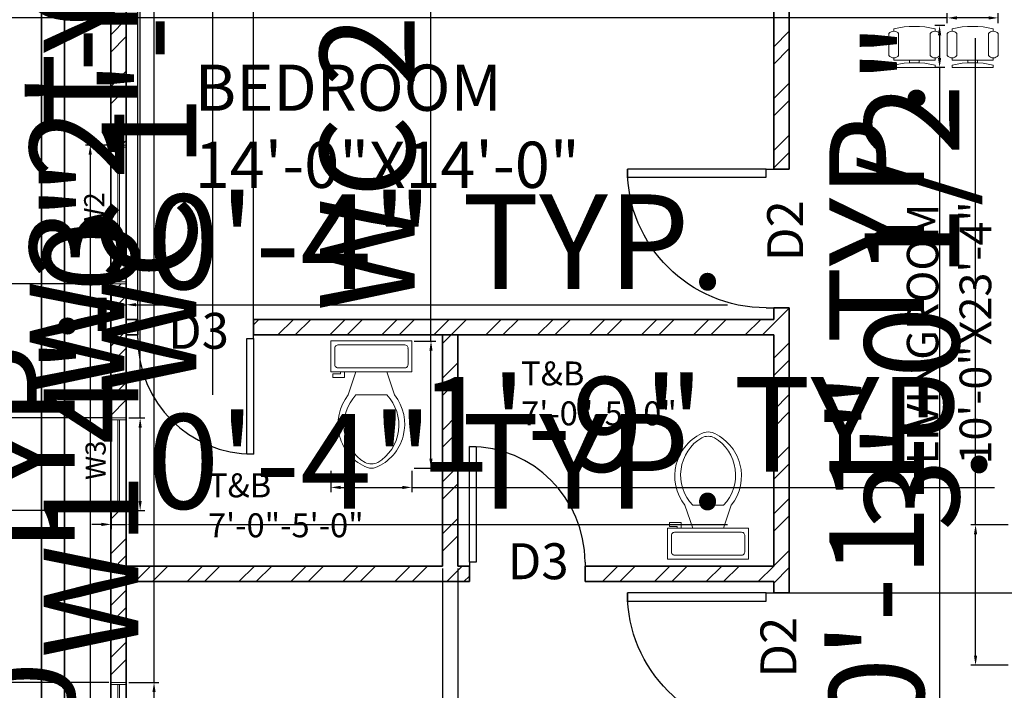
# Model space of a CAD drawing. Units: inches. Extents: x 1542 to 2523, y 1699 to 2449.
# Tile 3 of 7: x 1875 to 2130, y 1984 to 2158. Entities that reach past the tile are written whole.
import ezdxf

# ---------------------------------------------------------------- set-up
doc = ezdxf.new("R2010")
doc.units = ezdxf.units.IN
for name, color, linetype, lineweight in [('A-ANNO-DIMS', 7, 'Continuous', 18), ('A-ANNO-TEXT', 1, 'Continuous', 18), ('A-AREA-IDEN', 1, 'Continuous', 25), ('A-FLOR-FIXT', 9, 'Continuous', 18), ('A-WALL-PATT', 9, 'Continuous', 13), ('doors', 5, 'Continuous', 25), ('furniture', 9, 'Continuous', 18), ('walls', 7, 'Continuous', 35), ('windows', 93, 'Continuous', 18)]:
    doc.layers.add(name, color=color, linetype=linetype, lineweight=lineweight)
doc.styles.get("Standard").update_dxf_attribs({"font": 'arial.ttf'})
doc.dimstyles.new('ISO-25', dxfattribs={"dimtxt": 24.5625, "dimasz": 2.5, "dimexe": 1.25, "dimexo": 0.625, "dimtad": 1, "dimlunit": 4, "dimtxsty": 'Standard', "dimcen": 2.5, "dimadec": 0, "dimazin": 0, "dimtfac": 10, "dimtmove": 0, "dimatfit": 3, "dimfxl": 1, "dimarcsym": 0})

# ---------------------------------------------------------------- blocks, each defined once
blk = doc.blocks.new('*U2')
for p, q in [((0, 0), (0, -5)), ((30, 0), (30, -5))]:
    blk.add_line(p, q)
blk.add_lwpolyline([(0, 0), (0, 30), (1.75, 30), (1.75, 0)], close=True)
blk.add_arc((0, 0), 30, 0, 90)
blk = doc.blocks.new('Chair - Desk')
for p, q in [((-8.5, 0), (-8.5, -1)), ((-8.5, 0), (8.5, 0)), ((8.5, 0), (8.5, -1)), ((-8.5, -3), (-8.5, -4)), ((-8.5, -3), (8.5, -3)), ((-2, -3), (-2, -1.9355)), ((2, -1.9576), (2, -3)), ((8.5, -3), (8.5, -4)), ((-10.5, -5), (-10.5, -14)), ((-6.5, -14), (-6.5, -5)), ((6.5, -5), (6.5, -14)), ((10.5, -14), (10.5, -5)), ((-8.5, -15), (-8.5, -16)), ((8.5, -15), (8.5, -16))]:
    blk.add_line(p, q)
for centre, radius, start, end in [((-8.5, -6.5), 2.5, 36.8699, 143.1301), ((0, 34.625), 36.625, 256.5803, 283.4197), ((8.5, -6.5), 2.5, 36.8699, 143.1301), ((-8.5, -12.5), 2.5, 216.8699, 323.1301), ((0, 19.625), 36.625, 256.5803, 283.4197), ((8.5, -12.5), 2.5, 216.8699, 323.1301)]:
    blk.add_arc(centre, radius, start, end)
blk = doc.blocks.new('Toilet - top')
for p, q in [((9.5, -6), (9.5, -2)), ((-10, -8.5), (-8, -8.5)), ((-10, -9.5), (-10, -8.5)), ((-7, -9.5), (-10, -9.5)), ((-8, -8.5), (-8, -8)), ((-7, -8), (-7, -9.5)), ((-4, -8), (-6, -14)), ((4, -8), (6, -14)), ((4, -14), (-4, -14))]:
    blk.add_line(p, q)
blk.add_lwpolyline([(10.5, -8), (10.5, 0), (-10.5, 0), (-10.5, -8)], close=True)
for points in [[(-9.5, -2), (-9.5, -6)], [(8.5, -1), (-8.5, -1)], [(-8.5, -7), (8.5, -7)]]:
    blk.add_lwpolyline(points)
for centre, radius, start, end in [((-8.62, -1.88), 0.884, 81.8699, 188.1301), ((8.62, -1.88), 0.884, 351.8699, 98.1301), ((-8.62, -6.12), 0.884, 171.8699, 278.1301), ((8.62, -6.12), 0.884, 261.8699, 8.1301), ((3.52, -21.58), 12.17, 141.4691, 247.9714), ((4.2, -21.82), 11.33, 136.3677, 238.9468), ((-3.52, -21.58), 12.17, 292.0284, 38.5307), ((-4.2, -21.82), 11.33, 301.053, 43.6321), ((0, -27.88), 4, 245.7318, 294.2682), ((0, -29), 4, 254.8605, 285.1395)]:
    blk.add_arc(centre, radius, start, end)
blk = doc.blocks.new('WIN-W3-24IN')
for p, q in [((0, 0), (0, 24.03)), ((0, 24.03), (3.94, 24.03)), ((0, 23.53), (3.94, 23.53)), ((1.77, 0.5), (1.77, 23.53)), ((2.17, 0.5), (2.17, 23.53)), ((3.94, 24.03), (3.94, 0)), ((3.94, 0.5), (0, 0.5)), ((3.94, 0), (0, 0))]:
    blk.add_line(p, q)
blk = doc.blocks.new('WIN-W2-36IN')
for p, q in [((0, 3.94), (36.03, 3.94)), ((0, 0), (0, 3.94)), ((0.5, 0), (0.5, 3.94)), ((35.53, 3.94), (35.53, 0)), ((36.03, 3.94), (36.03, 0)), ((36.03, 0), (0, 0)), ((0.5, 2.17), (35.53, 2.17)), ((0.5, 1.77), (35.53, 1.77))]:
    blk.add_line(p, q)
blk = doc.blocks.new('WIN-W1-48IN')
for p, q in [((0, 0), (0, 48.03)), ((0, 48.03), (3.94, 48.03)), ((0, 47.53), (3.94, 47.53)), ((1.77, 0.5), (1.77, 47.53)), ((2.17, 0.5), (2.17, 47.53)), ((3.94, 48.03), (3.94, 0)), ((3.94, 0.5), (0, 0.5)), ((3.94, 0), (0, 0))]:
    blk.add_line(p, q)
blk = doc.blocks.new('*D26')
at = {"layer": 'A-ANNO-DIMS', "color": 0, "lineweight": -2, "transparency": 16777216}
for p, q in [((2115.34, 2158.69), (1845.86, 2158.69)), ((2115.34, 2157.33), (2115.34, 2159.94)), ((2126.05, 2158.69), (2117.84, 2158.69)), ((2128.55, 2157.33), (2128.55, 2159.94))]:
    blk.add_line(p, q, dxfattribs=at)
at = {"layer": 'A-ANNO-DIMS', "color": 0, "transparency": 16777216}
for points in [[(2117.84, 2159.1), (2117.84, 2158.27), (2115.34, 2158.69)], [(2126.05, 2159.1), (2126.05, 2158.27), (2128.55, 2158.69)]]:
    blk.add_solid(points, dxfattribs=at)
at = {"layer": 'Defpoints', "color": 0, "transparency": 16777216}
for p in [(2115.34, 2158.69), (2115.34, 2156.7), (2128.55, 2156.7)]:
    blk.add_point(p, dxfattribs=at)
at = {"layer": 'A-ANNO-DIMS', "color": 0, "transparency": 16777216, "insert": (1979.35, 2172.01), "char_height": 24.5625, "attachment_point": 5}
blk.add_mtext('CHAIR 1\'-1" TYP.', dxfattribs=at)
blk = doc.blocks.new('*D27')
at = {"layer": 'A-ANNO-DIMS', "color": 0, "lineweight": -2, "transparency": 16777216}
for p, q in [((2114.72, 2156.7), (2112.11, 2156.7)), ((2113.36, 2154.2), (2113.36, 2148.3)), ((2114.72, 2145.8), (2112.11, 2145.8)), ((2113.36, 2145.8), (2113.36, 1973.25))]:
    blk.add_line(p, q, dxfattribs=at)
at = {"layer": 'A-ANNO-DIMS', "color": 0, "transparency": 16777216}
for points in [[(2112.94, 2154.2), (2113.78, 2154.2), (2113.36, 2156.7)], [(2112.94, 2148.3), (2113.78, 2148.3), (2113.36, 2145.8)]]:
    blk.add_solid(points, dxfattribs=at)
at = {"layer": 'Defpoints', "color": 0, "transparency": 16777216}
for p in [(2115.34, 2156.7), (2113.36, 2145.8), (2115.34, 2145.8)]:
    blk.add_point(p, dxfattribs=at)
at = {"layer": 'A-ANNO-DIMS', "color": 0, "transparency": 16777216, "insert": (2100.19, 2058.28), "char_height": 24.5625, "attachment_point": 5, "rotation": 90}
blk.add_mtext('0\'-11" TYP.', dxfattribs=at)
blk = doc.blocks.new('*D28')
at = {"layer": 'A-ANNO-DIMS', "color": 0, "lineweight": -2, "transparency": 16777216}
for p, q in [((1905.99, 2054.87), (1905.99, 2270.35)), ((1903.01, 2054.87), (1907.24, 2054.87)), ((1905.99, 2033.33), (1905.99, 2052.37)), ((1903.01, 2030.83), (1907.24, 2030.83))]:
    blk.add_line(p, q, dxfattribs=at)
at = {"layer": 'A-ANNO-DIMS', "color": 0, "transparency": 16777216}
for points in [[(1905.57, 2052.37), (1906.4, 2052.37), (1905.99, 2054.87)], [(1905.57, 2033.33), (1906.4, 2033.33), (1905.99, 2030.83)]]:
    blk.add_solid(points, dxfattribs=at)
at = {"layer": 'Defpoints', "color": 0, "transparency": 16777216}
for p in [(1902.38, 2054.87), (1905.99, 2054.87), (1902.38, 2030.83)]:
    blk.add_point(p, dxfattribs=at)
at = {"layer": 'A-ANNO-DIMS', "color": 0, "transparency": 16777216, "insert": (1892.81, 2163.86), "char_height": 24.5625, "attachment_point": 5, "rotation": 90}
blk.add_mtext('W3 2\'-0" TYP.', dxfattribs=at)
blk = doc.blocks.new('*D29')
at = {"layer": 'A-ANNO-DIMS', "color": 0, "lineweight": -2, "transparency": 16777216}
for p, q in [((1898.45, 2030.21), (1898.45, 2025.98)), ((1902.38, 2030.21), (1902.38, 2025.98)), ((1895.95, 2027.23), (1893.45, 2027.23)), ((1898.45, 2027.23), (1902.38, 2027.23)), ((1904.88, 2027.23), (2058.35, 2027.23))]:
    blk.add_line(p, q, dxfattribs=at)
at = {"layer": 'A-ANNO-DIMS', "color": 0, "transparency": 16777216}
for points in [[(1895.95, 2027.65), (1895.95, 2026.81), (1898.45, 2027.23)], [(1904.88, 2027.65), (1904.88, 2026.81), (1902.38, 2027.23)]]:
    blk.add_solid(points, dxfattribs=at)
at = {"layer": 'Defpoints', "color": 0, "transparency": 16777216}
for p in [(1898.45, 2030.83), (1902.38, 2030.83), (1902.38, 2027.23)]:
    blk.add_point(p, dxfattribs=at)
at = {"layer": 'A-ANNO-DIMS', "color": 0, "transparency": 16777216, "insert": (1982.87, 2040.39), "char_height": 24.562, "attachment_point": 5}
blk.add_mtext('0\'-4" TYP.', dxfattribs=at)
blk = doc.blocks.new('*D30')
at = {"layer": 'A-ANNO-DIMS', "color": 0, "lineweight": -2, "transparency": 16777216}
for p, q in [((2181.19, 2203.89), (2176.38, 2203.89)), ((2177.63, 2201.39), (2177.63, 2178.49)), ((2181.19, 2175.99), (2176.38, 2175.99)), ((2177.63, 2175.99), (2177.63, 1878.93))]:
    blk.add_line(p, q, dxfattribs=at)
at = {"layer": 'A-ANNO-DIMS', "color": 0, "transparency": 16777216}
for points in [[(2177.21, 2201.39), (2178.05, 2201.39), (2177.63, 2203.89)], [(2177.21, 2178.49), (2178.05, 2178.49), (2177.63, 2175.99)]]:
    blk.add_solid(points, dxfattribs=at)
at = {"layer": 'Defpoints', "color": 0, "transparency": 16777216}
for p in [(2181.81, 2203.89), (2177.63, 2175.99), (2181.81, 2175.99)]:
    blk.add_point(p, dxfattribs=at)
at = {"layer": 'A-ANNO-DIMS', "color": 0, "transparency": 16777216, "insert": (2164.46, 2026.21), "char_height": 24.5625, "attachment_point": 5, "rotation": 90}
blk.add_mtext('TV UNIT 2\'-4" TYP.', dxfattribs=at)
blk = doc.blocks.new('*D32')
at = {"layer": 'A-ANNO-DIMS', "color": 0, "lineweight": -2, "transparency": 16777216}
for p, q in [((1922.46, 2274.54), (1926.04, 2274.54)), ((1924.79, 2272.04), (1924.79, 2257.33)), ((1922.46, 2254.83), (1926.04, 2254.83)), ((1924.79, 2254.83), (1924.79, 2060.84))]:
    blk.add_line(p, q, dxfattribs=at)
at = {"layer": 'A-ANNO-DIMS', "color": 0, "transparency": 16777216}
for points in [[(1924.37, 2272.04), (1925.21, 2272.04), (1924.79, 2274.54)], [(1924.37, 2257.33), (1925.21, 2257.33), (1924.79, 2254.83)]]:
    blk.add_solid(points, dxfattribs=at)
at = {"layer": 'Defpoints', "color": 0, "transparency": 16777216}
for p in [(1921.83, 2274.54), (1921.83, 2254.83), (1924.79, 2254.83)]:
    blk.add_point(p, dxfattribs=at)
at = {"layer": 'A-ANNO-DIMS', "color": 0, "transparency": 16777216, "insert": (1911.46, 2156.58), "char_height": 24.5625, "attachment_point": 5, "rotation": 90}
blk.add_mtext('WC 1\'-7 1/2"', dxfattribs=at)
blk = doc.blocks.new('*D34')
at = {"layer": 'A-ANNO-DIMS', "color": 0, "lineweight": -2, "transparency": 16777216}
for p, q in [((1981.43, 2074.83), (1981.43, 2296.01)), ((1977.09, 2074.83), (1982.68, 2074.83)), ((1981.43, 2044.29), (1981.43, 2072.33)), ((1977.09, 2041.79), (1982.68, 2041.79))]:
    blk.add_line(p, q, dxfattribs=at)
at = {"layer": 'A-ANNO-DIMS', "color": 0, "transparency": 16777216}
for points in [[(1981.01, 2072.33), (1981.84, 2072.33), (1981.43, 2074.83)], [(1981.01, 2044.29), (1981.84, 2044.29), (1981.43, 2041.79)]]:
    blk.add_solid(points, dxfattribs=at)
at = {"layer": 'Defpoints', "color": 0, "transparency": 16777216}
for p in [(1976.47, 2074.83), (1981.43, 2074.83), (1976.47, 2041.79)]:
    blk.add_point(p, dxfattribs=at)
at = {"layer": 'A-ANNO-DIMS', "color": 0, "transparency": 16777216, "insert": (1968.1, 2186.67), "char_height": 24.5625, "attachment_point": 5, "rotation": 90}
blk.add_mtext('WC 2\'-9" TYP.', dxfattribs=at)
blk = doc.blocks.new('*D35')
at = {"layer": 'A-ANNO-DIMS', "color": 0, "lineweight": -2, "transparency": 16777216}
for p, q in [((1955.47, 2041.16), (1955.47, 2035.58)), ((1976.47, 2041.16), (1976.47, 2035.58)), ((1957.97, 2036.83), (1973.97, 2036.83)), ((1976.47, 2036.83), (2127.63, 2036.83))]:
    blk.add_line(p, q, dxfattribs=at)
at = {"layer": 'A-ANNO-DIMS', "color": 0, "transparency": 16777216}
for points in [[(1957.97, 2037.25), (1957.97, 2036.41), (1955.47, 2036.83)], [(1973.97, 2037.25), (1973.97, 2036.41), (1976.47, 2036.83)]]:
    blk.add_solid(points, dxfattribs=at)
at = {"layer": 'Defpoints', "color": 0, "transparency": 16777216}
for p in [(1955.47, 2041.79), (1976.47, 2041.79), (1976.47, 2036.83)]:
    blk.add_point(p, dxfattribs=at)
at = {"layer": 'A-ANNO-DIMS', "color": 0, "transparency": 16777216, "insert": (2053.3, 2050), "char_height": 24.562, "attachment_point": 5}
blk.add_mtext('1\'-9" TYP.', dxfattribs=at)
blk = doc.blocks.new('*D36')
at = {"layer": 'A-ANNO-DIMS', "color": 0, "lineweight": -2, "transparency": 16777216}
for p, q in [((1897.82, 2125.68), (1891.79, 2125.68)), ((1893.04, 2123.18), (1893.04, 2092.15)), ((1897.82, 2089.65), (1891.79, 2089.65)), ((1893.04, 2089.65), (1893.04, 1874.17))]:
    blk.add_line(p, q, dxfattribs=at)
at = {"layer": 'A-ANNO-DIMS', "color": 0, "transparency": 16777216}
for points in [[(1892.62, 2123.18), (1893.46, 2123.18), (1893.04, 2125.68)], [(1892.62, 2092.15), (1893.46, 2092.15), (1893.04, 2089.65)]]:
    blk.add_solid(points, dxfattribs=at)
at = {"layer": 'Defpoints', "color": 0, "transparency": 16777216}
for p in [(1898.45, 2125.68), (1893.04, 2089.65), (1898.45, 2089.65)]:
    blk.add_point(p, dxfattribs=at)
at = {"layer": 'A-ANNO-DIMS', "color": 0, "transparency": 16777216, "insert": (1879.87, 1980.66), "char_height": 24.5625, "attachment_point": 5, "rotation": 90}
blk.add_mtext('W2 3\'-0" TYP.', dxfattribs=at)
blk = doc.blocks.new('*D37')
at = {"layer": 'A-ANNO-DIMS', "color": 0, "lineweight": -2, "transparency": 16777216}
for p, q in [((1898.45, 2089.02), (1898.45, 2082.99)), ((1902.38, 2089.02), (1902.38, 2082.99)), ((1895.95, 2084.24), (1893.45, 2084.24)), ((1898.45, 2084.24), (1902.38, 2084.24)), ((1904.88, 2084.24), (2058.35, 2084.24))]:
    blk.add_line(p, q, dxfattribs=at)
at = {"layer": 'A-ANNO-DIMS', "color": 0, "transparency": 16777216}
for points in [[(1895.95, 2084.66), (1895.95, 2083.83), (1898.45, 2084.24)], [(1904.88, 2084.66), (1904.88, 2083.83), (1902.38, 2084.24)]]:
    blk.add_solid(points, dxfattribs=at)
at = {"layer": 'Defpoints', "color": 0, "transparency": 16777216}
for p in [(1898.45, 2089.65), (1902.38, 2089.65), (1902.38, 2084.24)]:
    blk.add_point(p, dxfattribs=at)
at = {"layer": 'A-ANNO-DIMS', "color": 0, "transparency": 16777216, "insert": (1982.87, 2097.41), "char_height": 24.562, "attachment_point": 5}
blk.add_mtext('0\'-4" TYP.', dxfattribs=at)
blk = doc.blocks.new('*D40')
at = {"layer": 'A-ANNO-DIMS', "color": 0, "lineweight": -2, "transparency": 16777216}
for p, q in [((1909.59, 1986.22), (1909.59, 2201.7)), ((1903.01, 1986.22), (1910.84, 1986.22)), ((1909.59, 1940.69), (1909.59, 1983.72)), ((1903.01, 1938.19), (1910.84, 1938.19))]:
    blk.add_line(p, q, dxfattribs=at)
at = {"layer": 'A-ANNO-DIMS', "color": 0, "transparency": 16777216}
for points in [[(1909.17, 1983.72), (1910, 1983.72), (1909.59, 1986.22)], [(1909.17, 1940.69), (1910, 1940.69), (1909.59, 1938.19)]]:
    blk.add_solid(points, dxfattribs=at)
at = {"layer": 'Defpoints', "color": 0, "transparency": 16777216}
for p in [(1902.38, 1986.22), (1909.59, 1986.22), (1902.38, 1938.19)]:
    blk.add_point(p, dxfattribs=at)
at = {"layer": 'A-ANNO-DIMS', "color": 0, "transparency": 16777216, "insert": (1896.42, 2095.21), "char_height": 24.5625, "attachment_point": 5, "rotation": 90}
blk.add_mtext('W1 4\'-0" TYP.', dxfattribs=at)
blk = doc.blocks.new('*D43')
at = {"layer": 'A-ANNO-DIMS', "color": 0, "lineweight": -2, "transparency": 16777216}
for p, q in [((2122.69, 2027.16), (2122.69, 2153.42)), ((2131.12, 2027.16), (2121.44, 2027.16)), ((2122.69, 1993.17), (2122.69, 2024.66)), ((2131.12, 1990.67), (2121.44, 1990.67))]:
    blk.add_line(p, q, dxfattribs=at)
at = {"layer": 'A-ANNO-DIMS', "color": 0, "transparency": 16777216}
for points in [[(2122.28, 2024.66), (2123.11, 2024.66), (2122.69, 2027.16)], [(2122.28, 1993.17), (2123.11, 1993.17), (2122.69, 1990.67)]]:
    blk.add_solid(points, dxfattribs=at)
at = {"layer": 'Defpoints', "color": 0, "transparency": 16777216}
for p in [(2122.69, 2027.16), (2131.75, 2027.16), (2131.75, 1990.67)]:
    blk.add_point(p, dxfattribs=at)
at = {"layer": 'A-ANNO-DIMS', "color": 0, "transparency": 16777216, "insert": (2109.36, 2091.54), "char_height": 24.562, "attachment_point": 5, "rotation": 90}
blk.add_mtext('3\'-0 1/2"', dxfattribs=at)
blk = doc.blocks.new('*D47')
at = {"layer": 'A-ANNO-DIMS', "color": 0, "lineweight": -2, "transparency": 16777216}
for p, q in [((2268.83, 2009.44), (2268.83, 2078.47)), ((2071.01, 2009.44), (2270.08, 2009.44)), ((2268.83, 1975.94), (2268.83, 2006.94)), ((2071.01, 1973.44), (2270.08, 1973.44))]:
    blk.add_line(p, q, dxfattribs=at)
at = {"layer": 'A-ANNO-DIMS', "color": 0, "transparency": 16777216}
for points in [[(2268.42, 2006.94), (2269.25, 2006.94), (2268.83, 2009.44)], [(2268.42, 1975.94), (2269.25, 1975.94), (2268.83, 1973.44)]]:
    blk.add_solid(points, dxfattribs=at)
at = {"layer": 'Defpoints', "color": 0, "transparency": 16777216}
for p in [(2070.38, 2009.44), (2268.83, 2009.44), (2070.38, 1973.44)]:
    blk.add_point(p, dxfattribs=at)
at = {"layer": 'A-ANNO-DIMS', "color": 0, "transparency": 16777216, "insert": (2255.66, 2045.2), "char_height": 24.562, "attachment_point": 5, "rotation": 90}
blk.add_mtext('3\'-0"', dxfattribs=at)
blk = doc.blocks.new('*D48')
at = {"layer": 'A-ANNO-DIMS', "color": 0, "lineweight": -2, "transparency": 16777216}
for p, q in [((1905.38, 2077.06), (1905.38, 2320.14)), ((1935.38, 2077.06), (1935.38, 2320.14)), ((1907.88, 2318.89), (1932.88, 2318.89)), ((1935.38, 2318.89), (2004.84, 2318.89))]:
    blk.add_line(p, q, dxfattribs=at)
at = {"layer": 'A-ANNO-DIMS', "color": 0, "transparency": 16777216}
for points in [[(1907.88, 2319.31), (1907.88, 2318.47), (1905.38, 2318.89)], [(1932.88, 2319.31), (1932.88, 2318.47), (1935.38, 2318.89)]]:
    blk.add_solid(points, dxfattribs=at)
at = {"layer": 'Defpoints', "color": 0, "transparency": 16777216}
for p in [(1935.38, 2318.89), (1905.38, 2076.44), (1935.38, 2076.44)]:
    blk.add_point(p, dxfattribs=at)
at = {"layer": 'A-ANNO-DIMS', "color": 0, "transparency": 16777216, "insert": (1971.36, 2332.05), "char_height": 24.562, "attachment_point": 5}
blk.add_mtext('2\'-6"', dxfattribs=at)
blk = doc.blocks.new('*D49')
at = {"layer": 'A-ANNO-DIMS', "color": 0, "lineweight": -2, "transparency": 16777216}
for p, q in [((1851.93, 1958.44), (1851.93, 2027.9)), ((2157.76, 1958.44), (1850.68, 1958.44)), ((1851.93, 1936.94), (1851.93, 1955.94)), ((2157.76, 1934.44), (1850.68, 1934.44))]:
    blk.add_line(p, q, dxfattribs=at)
at = {"layer": 'A-ANNO-DIMS', "color": 0, "transparency": 16777216}
for points in [[(1851.52, 1955.94), (1852.35, 1955.94), (1851.93, 1958.44)], [(1851.52, 1936.94), (1852.35, 1936.94), (1851.93, 1934.44)]]:
    blk.add_solid(points, dxfattribs=at)
at = {"layer": 'Defpoints', "color": 0, "transparency": 16777216}
for p in [(1851.93, 1958.44), (2158.38, 1958.44), (2158.38, 1934.44)]:
    blk.add_point(p, dxfattribs=at)
at = {"layer": 'A-ANNO-DIMS', "color": 0, "transparency": 16777216, "insert": (1838.77, 1994.42), "char_height": 24.562, "attachment_point": 5, "rotation": 90}
blk.add_mtext('2\'-0"', dxfattribs=at)
blk = doc.blocks.new('*D56')
at = {"layer": 'A-ANNO-DIMS', "color": 0, "lineweight": -2, "transparency": 16777216}
for p, q in [((1851.93, 2030.83), (1851.93, 2157.09)), ((1897.82, 2030.83), (1850.68, 2030.83)), ((1851.93, 1988.72), (1851.93, 2028.33)), ((1897.82, 1986.22), (1850.68, 1986.22))]:
    blk.add_line(p, q, dxfattribs=at)
at = {"layer": 'A-ANNO-DIMS', "color": 0, "transparency": 16777216}
for points in [[(1851.52, 2028.33), (1852.35, 2028.33), (1851.93, 2030.83)], [(1851.52, 1988.72), (1852.35, 1988.72), (1851.93, 1986.22)]]:
    blk.add_solid(points, dxfattribs=at)
at = {"layer": 'Defpoints', "color": 0, "transparency": 16777216}
for p in [(1851.93, 2030.83), (1898.45, 2030.83), (1898.45, 1986.22)]:
    blk.add_point(p, dxfattribs=at)
at = {"layer": 'A-ANNO-DIMS', "color": 0, "transparency": 16777216, "insert": (1838.6, 2095.21), "char_height": 24.562, "attachment_point": 5, "rotation": 90}
blk.add_mtext('3\'-8 1/2"', dxfattribs=at)
blk = doc.blocks.new('*D57')
at = {"layer": 'A-ANNO-DIMS', "color": 0, "lineweight": -2, "transparency": 16777216}
for p, q in [((1851.93, 2089.65), (1851.93, 2178.19)), ((1897.82, 2089.65), (1850.68, 2089.65)), ((1851.93, 2057.37), (1851.93, 2087.15)), ((1897.82, 2054.87), (1850.68, 2054.87))]:
    blk.add_line(p, q, dxfattribs=at)
at = {"layer": 'A-ANNO-DIMS', "color": 0, "transparency": 16777216}
for points in [[(1851.52, 2087.15), (1852.35, 2087.15), (1851.93, 2089.65)], [(1851.52, 2057.37), (1852.35, 2057.37), (1851.93, 2054.87)]]:
    blk.add_solid(points, dxfattribs=at)
at = {"layer": 'Defpoints', "color": 0, "transparency": 16777216}
for p in [(1851.93, 2089.65), (1898.45, 2089.65), (1898.45, 2054.87)]:
    blk.add_point(p, dxfattribs=at)
at = {"layer": 'A-ANNO-DIMS', "color": 0, "transparency": 16777216, "insert": (1838.98, 2135.17), "char_height": 24.562, "attachment_point": 5, "rotation": 90}
blk.add_mtext('2\'-11"', dxfattribs=at)
blk = doc.blocks.new('*D67')
at = {"layer": 'A-ANNO-DIMS', "color": 0, "lineweight": -2, "transparency": 16777216}
for p, q in [((1984.38, 2015.81), (1984.38, 1720.74)), ((1902.38, 2011.81), (1902.38, 1720.74)), ((1904.88, 1721.99), (1981.88, 1721.99)), ((1984.38, 1721.99), (2072.64, 1721.99))]:
    blk.add_line(p, q, dxfattribs=at)
at = {"layer": 'A-ANNO-DIMS', "color": 0, "transparency": 16777216}
for points in [[(1904.88, 1722.41), (1904.88, 1721.57), (1902.38, 1721.99)], [(1981.88, 1722.41), (1981.88, 1721.57), (1984.38, 1721.99)]]:
    blk.add_solid(points, dxfattribs=at)
at = {"layer": 'Defpoints', "color": 0, "transparency": 16777216}
for p in [(1984.38, 2016.44), (1902.38, 2012.44), (1984.38, 1721.99)]:
    blk.add_point(p, dxfattribs=at)
at = {"layer": 'A-ANNO-DIMS', "color": 0, "transparency": 16777216, "insert": (2029.76, 1735.15), "char_height": 24.562, "attachment_point": 5}
blk.add_mtext('6\'-10"', dxfattribs=at)
blk = doc.blocks.new('*D68')
at = {"layer": 'A-ANNO-DIMS', "color": 0, "lineweight": -2, "transparency": 16777216}
for p, q in [((1984.38, 2015.81), (1984.38, 1720.74)), ((1988.38, 2015.81), (1988.38, 1720.74)), ((1981.88, 1721.99), (1979.38, 1721.99)), ((1984.38, 1721.99), (1988.38, 1721.99)), ((1990.88, 1721.99), (2059.93, 1721.99))]:
    blk.add_line(p, q, dxfattribs=at)
at = {"layer": 'A-ANNO-DIMS', "color": 0, "transparency": 16777216}
for points in [[(1981.88, 1722.41), (1981.88, 1721.57), (1984.38, 1721.99)], [(1990.88, 1722.41), (1990.88, 1721.57), (1988.38, 1721.99)]]:
    blk.add_solid(points, dxfattribs=at)
at = {"layer": 'Defpoints', "color": 0, "transparency": 16777216}
for p in [(1984.38, 2016.44), (1988.38, 2016.44), (1988.38, 1721.99)]:
    blk.add_point(p, dxfattribs=at)
at = {"layer": 'A-ANNO-DIMS', "color": 0, "transparency": 16777216, "insert": (2026.65, 1735.15), "char_height": 24.562, "attachment_point": 5}
blk.add_mtext('0\'-4"', dxfattribs=at)
blk = doc.blocks.new('*D69')
at = {"layer": 'A-ANNO-DIMS', "color": 0, "lineweight": -2, "transparency": 16777216}
for p, q in [((1902.38, 2077.06), (1902.38, 2320.14)), ((1905.38, 2077.06), (1905.38, 2320.14)), ((1899.88, 2318.89), (1897.38, 2318.89)), ((1902.38, 2318.89), (1905.38, 2318.89)), ((1907.88, 2318.89), (1976.93, 2318.89))]:
    blk.add_line(p, q, dxfattribs=at)
at = {"layer": 'A-ANNO-DIMS', "color": 0, "transparency": 16777216}
for points in [[(1899.88, 2319.31), (1899.88, 2318.47), (1902.38, 2318.89)], [(1907.88, 2319.31), (1907.88, 2318.47), (1905.38, 2318.89)]]:
    blk.add_solid(points, dxfattribs=at)
at = {"layer": 'Defpoints', "color": 0, "transparency": 16777216}
for p in [(1905.38, 2318.89), (1902.38, 2076.44), (1905.38, 2076.44)]:
    blk.add_point(p, dxfattribs=at)
at = {"layer": 'A-ANNO-DIMS', "color": 0, "transparency": 16777216, "insert": (1943.65, 2332.06), "char_height": 24.562, "attachment_point": 5}
blk.add_mtext('0\'-3"', dxfattribs=at)

msp = doc.modelspace()

# ---------------------------------------------------------------- hatches: boundary and pattern name
at = {"layer": 'A-WALL-PATT'}
h = msp.add_hatch(dxfattribs=at)
h.set_pattern_fill('ANSI32', color=256)
h.paths.add_polyline_path([(1902.383, 2125.681), (1898.383, 2125.681), (1898.383, 2252.439), (2030.138, 2252.439), (2030.138, 2248.439), (1902.383, 2248.439)])
h = msp.add_hatch(dxfattribs=at)
h.set_pattern_fill('ANSI32', color=256)
h.paths.add_polyline_path([(2074.383, 2248.439), (2070.383, 2248.439), (2070.383, 2119.439), (2074.383, 2119.439)])
h = msp.add_hatch(dxfattribs=at)
h.set_pattern_fill('ANSI32', color=256)
h.paths.add_polyline_path([(1902.383, 2089.649), (1898.383, 2089.649), (1898.383, 2054.866), (1902.383, 2054.866)])
h = msp.add_hatch(dxfattribs=at)
h.set_pattern_fill('ANSI32', color=256)
h.paths.add_polyline_path([(2074.383, 2083.439), (2070.383, 2083.439), (2070.383, 2080.439), (1935.383, 2080.439), (1935.383, 2076.439), (2070.383, 2076.439), (2070.383, 2016.439), (2021.383, 2016.439), (2021.383, 2012.439), (2070.383, 2012.439), (2070.383, 2009.439), (2074.383, 2009.439), (2074.383, 2012.439)])
h = msp.add_hatch(dxfattribs=at)
h.set_pattern_fill('ANSI32', color=256)
h.paths.add_polyline_path([(1905.383, 2080.439), (1902.383, 2080.439), (1902.383, 2076.439), (1905.383, 2076.439)])
h = msp.add_hatch(dxfattribs=at)
h.set_pattern_fill('ANSI32', color=256)
h.paths.add_polyline_path([(1988.383, 2076.439), (1984.383, 2076.439), (1984.383, 2016.439), (1902.383, 2016.439), (1902.383, 2012.439), (1991.383, 2012.439), (1991.383, 2016.439), (1988.383, 2016.439)])
h = msp.add_hatch(dxfattribs=at)
h.set_pattern_fill('ANSI32', color=256)
h.paths.add_polyline_path([(1902.383, 2030.833), (1898.383, 2030.833), (1898.383, 1986.223), (1902.383, 1986.223)])

# ---------------------------------------------------------------- linework, layer by layer
at = {"layer": 'walls'}
for p, q in [((1880.383, 1750.439), (1880.383, 2290.439)), ((1886.383, 1756.439), (1886.383, 2284.439)), ((1898.383, 1840.439), (1898.383, 2252.439)), ((1902.383, 1844.439), (1902.383, 2248.439)), ((2070.383, 2119.439), (2070.383, 2248.439)), ((2074.383, 2119.439), (2074.383, 2248.439)), ((2070.383, 2119.439), (2074.383, 2119.439)), ((2074.383, 2083.439), (2070.383, 2083.439)), ((2070.383, 2080.439), (2070.383, 2083.439)), ((2074.383, 2080.439), (2074.383, 2083.439)), ((2074.383, 2009.439), (2074.383, 2083.439)), ((1902.383, 2080.439), (1905.383, 2080.439)), ((1905.383, 2080.439), (1902.383, 2080.439)), ((1905.383, 2080.439), (1905.383, 2076.439)), ((2070.383, 2080.439), (1935.383, 2080.439)), ((1935.383, 2076.439), (1935.383, 2080.439)), ((1905.383, 2076.439), (1902.383, 2076.439)), ((2070.383, 2076.439), (1935.383, 2076.439)), ((1984.383, 2016.439), (1984.383, 2076.439)), ((1988.383, 2016.439), (1988.383, 2076.439)), ((2070.383, 2016.439), (2070.383, 2076.439)), ((1984.383, 2016.439), (1902.383, 2016.439)), ((1988.383, 2016.439), (1991.383, 2016.439)), ((1991.383, 2016.439), (1988.383, 2016.439)), ((1991.383, 2016.439), (1991.383, 2012.439)), ((2070.383, 2016.439), (2021.383, 2016.439)), ((2021.383, 2012.439), (2021.383, 2016.439)), ((1991.383, 2012.439), (1902.383, 2012.439)), ((2070.383, 2012.439), (2021.383, 2012.439)), ((2070.383, 2009.439), (2070.383, 2012.439)), ((2074.383, 2012.439), (2074.383, 2009.439)), ((2074.383, 2009.439), (2070.383, 2009.439))]:
    msp.add_line(p, q, dxfattribs=at)

# ---------------------------------------------------------------- block references
at = {"layer": 'A-FLOR-FIXT'}
msp.add_blockref('Toilet - top', (1965.969, 2074.834), dxfattribs=at)
at = {"layer": 'A-FLOR-FIXT', "xscale": -1, "rotation": 180}
msp.add_blockref('Toilet - top', (2053.318, 2018.218), dxfattribs=at)
at = {"layer": 'doors', "xscale": -1.199999999999999, "yscale": 1.199999999999999, "zscale": 1.199999999999999, "rotation": 90}
for p in [(2068.383, 2119.439), (2068.383, 2009.439)]:
    msp.add_blockref('*U2', p, dxfattribs=at)
at = {"layer": 'doors', "rotation": 180}
msp.add_blockref('*U2', (1935.383, 2075.439), dxfattribs=at)
at = {"layer": 'doors'}
msp.add_blockref('*U2', (1991.383, 2017.439), dxfattribs=at)
at = {"layer": 'furniture', "xscale": 0.6288640780466365, "yscale": 0.6288640780466365, "zscale": 0.6288640780466365, "rotation": 180}
for p in [(2106.83, 2145.804), (2121.944, 2145.804)]:
    msp.add_blockref('Chair - Desk', p, dxfattribs=at)
at = {"layer": 'windows', "rotation": 269.9999999999994}
msp.add_blockref('WIN-W2-36IN', (1898.446, 2125.681), dxfattribs=at)
at = {"layer": 'windows'}
for name, p in [('WIN-W3-24IN', (1898.446, 2030.833)), ('WIN-W1-48IN', (1898.446, 1938.191))]:
    msp.add_blockref(name, p, dxfattribs=at)

# ---------------------------------------------------------------- texts
at = {"layer": 'A-ANNO-TEXT', "attachment_point": 1, "rotation": 90}
for s, width, gutter_width, insert, char_height in [('W2', 1.62225, 26.164, (1891.453, 2103.206), 5.2329), ('D2', 3.38383, 46.636, (2068.636, 2095.552), 9.3273), ('W3', 1.62225, 26.164, (1891.814, 2038.757), 5.2329), ('D2', 3.38383, 46.636, (2066.897, 1987.446), 9.3273)]:
    msp.add_mtext_dynamic_manual_height_columns(s, width=width, gutter_width=gutter_width, heights=[0], dxfattribs=dict(at, insert=insert, char_height=char_height))
at = {"layer": 'A-ANNO-TEXT', "char_height": 9.3273, "attachment_point": 1}
for insert in [(1913.207, 2082.137), (2001.315, 2022.338)]:
    msp.add_mtext_dynamic_manual_height_columns('D3', width=3.38383, gutter_width=46.636, heights=[0], dxfattribs=dict(at, insert=insert))
at = {"layer": 'A-AREA-IDEN', "attachment_point": 1}
for s, width, gutter_width, insert, char_height in [('BEDROOM\\P14\'-0"X14\'-0"', 0.33006, 12.5, (1920.138, 2146.57), 12), ('T&B\\P7\'-0"-5\'-0"', 2.21048, 31.072, (2004.805, 2069.517), 6.21441), ('T&B\\P7\'-0"-5\'-0"', 2.21048, 31.072, (1923.572, 2040.47), 6.21441)]:
    msp.add_mtext_dynamic_manual_height_columns(s, width=width, gutter_width=gutter_width, heights=[0], dxfattribs=dict(at, insert=insert, char_height=char_height))
at = {"layer": 'A-AREA-IDEN', "insert": (2104.866, 2042.778), "char_height": 8.20997, "attachment_point": 1, "rotation": 90}
msp.add_mtext_dynamic_manual_height_columns('LIVINGROOM\\P10\'-0"X23\'-4"', width=0.22582, gutter_width=8.552, heights=[0], dxfattribs=at)

# ---------------------------------------------------------------- dimensions: what is measured, and where the dimension line sits
at = {"layer": 'A-ANNO-DIMS'}
for base, p1, p2, picture, middle in [((1905.383, 2318.889), (1902.383, 2076.439), (1905.383, 2076.439), '*D69', (1943.654, 2332.063)), ((1935.383, 2318.889), (1905.383, 2076.439), (1935.383, 2076.439), '*D48', (1971.364, 2332.055)), ((1984.383, 1721.989), (1902.383, 2012.439), (1984.383, 2016.439), '*D67', (2029.763, 1735.155)), ((1988.383, 1721.989), (1984.383, 2016.439), (1988.383, 2016.439), '*D68', (2026.654, 1735.155))]:
    dim = msp.add_linear_dim(base=base, p1=p1, p2=p2, dimstyle='ISO-25', override={"dimdec": 1, "dimlfac": 1, "dimrnd": 0, "dimzin": 1, "dimdsep": 46, "dimlunit": 4, "dimfrac": 2}, dxfattribs=at)
    dim.commit()
    dim.dimension.update_dxf_attribs({"geometry": picture, "text_midpoint": middle})
for base, p1, p2, angle, text, picture, middle in [((1981.426, 2074.834), (1976.469, 2041.788), (1976.469, 2074.834), 90, 'WC <> TYP.', '*D34', (1968.101, 2186.673)), ((1924.788, 2254.826), (1921.831, 2274.545), (1921.831, 2254.826), 270, 'WC <>', '*D32', (1911.463, 2156.584)), ((1905.987, 2054.866), (1902.383, 2030.833), (1902.383, 2054.866), 90, 'W3 <> TYP.', '*D28', (1892.813, 2163.856)), ((2115.34, 2158.686), (2128.547, 2156.705), (2115.34, 2156.705), 180, 'CHAIR <> TYP.', '*D26', (1979.35, 2172.011)), ((1909.587, 1986.223), (1902.383, 1938.191), (1902.383, 1986.223), 90, 'W1 <> TYP.', '*D40', (1896.422, 2095.213)), ((2177.629, 2175.993), (2181.813, 2203.885), (2181.813, 2175.993), 270, 'TV UNIT <> TYP.', '*D30', (2164.463, 2026.213)), ((2113.36, 2145.804), (2115.34, 2156.705), (2115.34, 2145.804), 270, '<> TYP.', '*D27', (2100.194, 2058.277)), ((1893.041, 2089.649), (1898.446, 2125.681), (1898.446, 2089.649), 270, 'W2 <> TYP.', '*D36', (1879.867, 1980.659))]:
    dim = msp.add_linear_dim(base=base, p1=p1, p2=p2, angle=angle, text=text, dimstyle='ISO-25', override={"dimdec": 1, "dimlfac": 1, "dimrnd": 0, "dimzin": 1, "dimdsep": 46, "dimlunit": 4, "dimfrac": 2}, dxfattribs=at)
    dim.commit()
    dim.dimension.update_dxf_attribs({"geometry": picture, "text_midpoint": middle})
for base, p1, p2, picture, middle in [((1851.933, 2089.649), (1898.446, 2054.866), (1898.446, 2089.649), '*D57', (1838.976, 2135.172)), ((1851.933, 2030.833), (1898.446, 1986.223), (1898.446, 2030.833), '*D56', (1838.599, 2095.214)), ((2122.695, 2027.16), (2131.75, 1990.673), (2131.75, 2027.16), '*D43', (2109.361, 2091.54)), ((2268.833, 2009.439), (2070.383, 1973.439), (2070.383, 2009.439), '*D47', (2255.658, 2045.202)), ((1851.933, 1958.439), (2158.383, 1934.439), (2158.383, 1958.439), '*D49', (1838.767, 1994.42))]:
    dim = msp.add_linear_dim(base=base, p1=p1, p2=p2, angle=90, dimstyle='ISO-25', override={"dimdec": 1, "dimlfac": 1, "dimrnd": 0, "dimzin": 1, "dimdsep": 46, "dimlunit": 4, "dimfrac": 2}, dxfattribs=at)
    dim.commit()
    dim.dimension.update_dxf_attribs({"geometry": picture, "text_midpoint": middle})
for base, p1, p2, picture, middle in [((1902.383, 2084.244), (1898.446, 2089.649), (1902.383, 2089.649), '*D37', (1982.868, 2097.41)), ((1976.469, 2036.831), (1955.469, 2041.788), (1976.469, 2041.788), '*D35', (2053.298, 2049.997)), ((1902.383, 2027.229), (1898.446, 2030.833), (1902.383, 2030.833), '*D29', (1982.868, 2040.395))]:
    dim = msp.add_linear_dim(base=base, p1=p1, p2=p2, text='<> TYP.', dimstyle='ISO-25', override={"dimdec": 1, "dimlfac": 1, "dimrnd": 0, "dimzin": 1, "dimdsep": 46, "dimlunit": 4, "dimfrac": 2}, dxfattribs=at)
    dim.commit()
    dim.dimension.update_dxf_attribs({"geometry": picture, "text_midpoint": middle})

doc.saveas('drawing.dxf')
